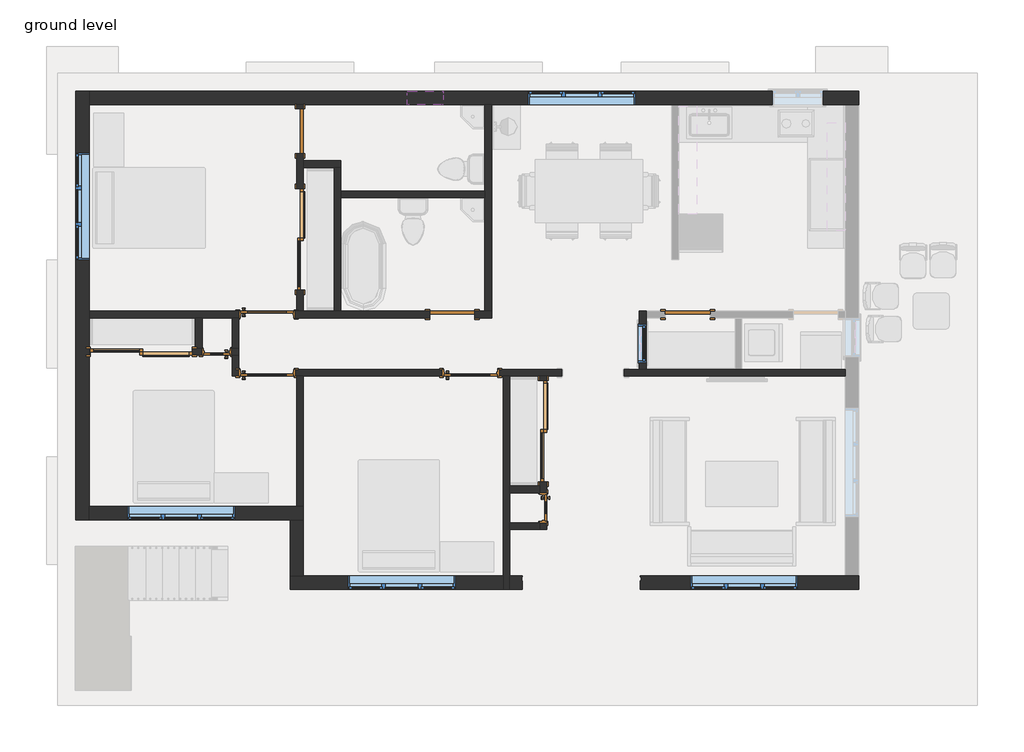
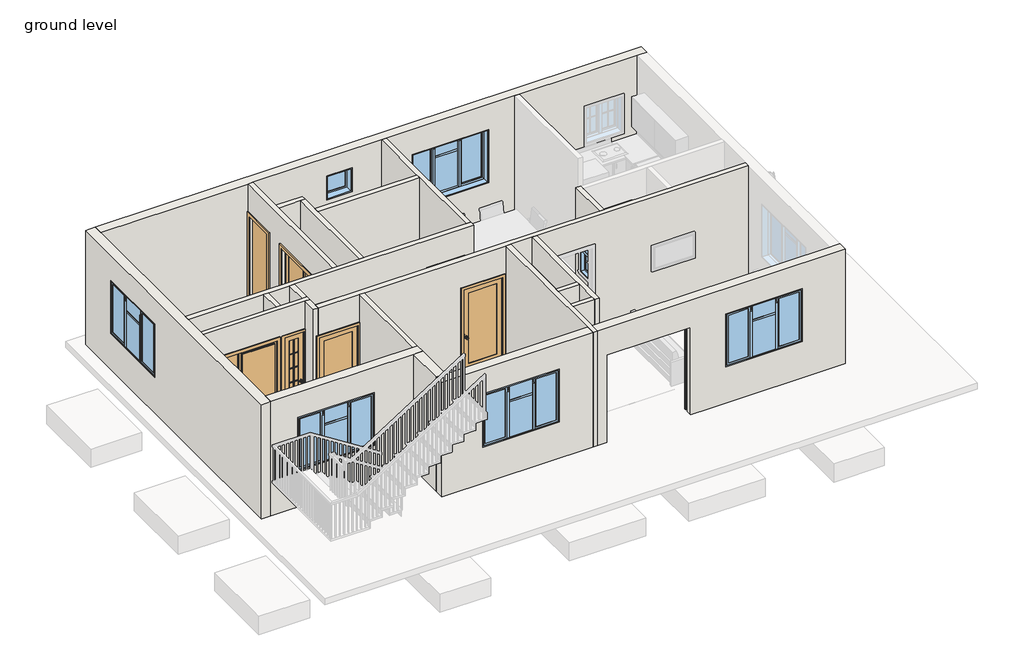
# One storey, part 1 of 4: 23 walls, 11 doors, 7 windows.
"""IFC4 building model written with IfcOpenShell, lengths in millimetres."""

from ifc_helpers import new_model, si_unit, frame, origin, place, context, project, spatial, polyline, outline, extrude, faceted_brep, transform, mapped, element, save
from components import door_505787c2, door_a3feeac7, door_3c6ab76a, door_ccf0cbd1, door_214872d5, door_78caadf7, window_80340324, window_7a1f68bc, window_d2058a86

model = new_model("IFC4")

# Units and contexts
model_context = context("Model", 3, world=origin())
ifc_project = project(units=[si_unit("LENGTHUNIT", "METRE", prefix="MILLI")], contexts=[model_context])

# Site, building, storey
site = spatial("IfcSite", under=ifc_project)
building = spatial("IfcBuilding", under=site)
storey = spatial("IfcBuildingStorey", under=building, Name="ground level", Elevation=609.6)

# Doors
placement = place(None, origin())
door_shape = door_505787c2(model_context)
element("IfcDoor", 1, ObjectType="Door-Double-Sliding : 68\" x 84\"", at=placement, inside=storey, context=model_context, shape_type="MappedRepresentation", body=[
    mapped(door_shape, transform((-1350.0263529, 910.5161978, 609.6), x_axis=(0.0, -1.0, 0.0), y_axis=(1.0, 0.0, 0.0), z_axis=(0.0, 0.0, 1.0))),
])
element("IfcDoor", 2, ObjectType="Door-Double-Sliding : 68\" x 84\"", at=placement, inside=storey, context=model_context, shape_type="MappedRepresentation", body=[
    mapped(door_shape, transform((-8046.1013529, 2383.7161978, 609.6), x_axis=(-1.0, 0.0, 0.0), y_axis=(0.0, -1.0, 0.0), z_axis=(0.0, 0.0, 1.0))),
])
element("IfcDoor", 3, ObjectType="Door-Double-Sliding : 68\" x 84\"", at=placement, inside=storey, context=model_context, shape_type="MappedRepresentation", body=[
    mapped(door_shape, transform((-5477.5263529, 4168.0661978, 609.6), x_axis=(0.0, -1.0, 0.0), y_axis=(1.0, 0.0, 0.0), z_axis=(0.0, 0.0, 1.0))),
])
door_2_shape = door_a3feeac7(model_context)
element("IfcDoor", 4, ObjectType="Door-Interior-Single-1_Panel-Wood : 36\" x 84\"", at=placement, inside=storey, context=model_context, shape_type="MappedRepresentation", body=[
    mapped(door_2_shape, transform((-5912.5013529, 1897.9411978, 609.6), x_axis=(1.0, 0.0, 0.0), y_axis=(0.0, 1.0, 0.0), z_axis=(0.0, 0.0, 1.0))),
])
element("IfcDoor", 5, ObjectType="Door-Interior-Single-1_Panel-Wood : 36\" x 84\"", at=placement, inside=storey, context=model_context, shape_type="MappedRepresentation", body=[
    mapped(door_2_shape, transform((-2454.9263529, 1897.9411978, 609.6), x_axis=(1.0, 0.0, 0.0), y_axis=(0.0, 1.0, 0.0), z_axis=(0.0, 0.0, 1.0))),
])
door_3_shape = door_3c6ab76a(model_context)
element("IfcDoor", 6, ObjectType="Door-Interior-Single-1_Panel-Wood : 36\" x 84\"", at=placement, inside=storey, context=model_context, shape_type="MappedRepresentation", body=[
    mapped(door_3_shape, transform((-5912.5013529, 2894.8911978, 609.6), x_axis=(1.0, 0.0, 0.0), y_axis=(0.0, 1.0, 0.0), z_axis=(0.0, 0.0, 1.0))),
])
door_4_shape = door_ccf0cbd1(model_context)
element("IfcDoor", 7, ObjectType="Door-Interior-Single-Full Glass-Wood : 18\" x 84\"", at=placement, inside=storey, context=model_context, shape_type="MappedRepresentation", body=[
    mapped(door_4_shape, transform((-1219.8513529, -391.2338022, 609.6), x_axis=(0.0, -1.0, 0.0), y_axis=(1.0, 0.0, 0.0), z_axis=(0.0, 0.0, 1.0))),
])
element("IfcDoor", 8, ObjectType="Door-Interior-Single-Full Glass-Wood : 18\" x 84\"", at=placement, inside=storey, context=model_context, shape_type="MappedRepresentation", body=[
    mapped(door_4_shape, transform((-6766.5763529, 2253.5411978, 609.6), x_axis=(-1.0, 0.0, 0.0), y_axis=(0.0, -1.0, 0.0), z_axis=(0.0, 0.0, 1.0))),
])
door_5_shape = door_214872d5(model_context)
element("IfcDoor", 9, ObjectType="Single-Flush : 30\" x 84\"", at=placement, inside=storey, context=model_context, shape_type="MappedRepresentation", body=[
    mapped(door_5_shape, transform((-2766.0763529, 2891.7161978, 609.6), x_axis=(1.0, 0.0, 0.0), y_axis=(0.0, 1.0, 0.0), z_axis=(0.0, 0.0, 1.0))),
])
element("IfcDoor", 10, ObjectType="Single-Flush : 30\" x 84\"", at=placement, inside=storey, context=model_context, shape_type="MappedRepresentation", body=[
    mapped(door_5_shape, transform((1228.0736471, 2891.7161978, 609.6), x_axis=(1.0, 0.0, 0.0), y_axis=(0.0, 1.0, 0.0), z_axis=(0.0, 0.0, 1.0))),
])
door_6_shape = door_78caadf7(model_context)
element("IfcDoor", 11, ObjectType="Single-Flush : 30\" x 84\"", at=placement, inside=storey, context=model_context, shape_type="MappedRepresentation", body=[
    mapped(door_6_shape, transform((-5350.5263529, 6006.3911978, 609.6), x_axis=(0.0, 1.0, 0.0), y_axis=(-1.0, 0.0, 0.0), z_axis=(0.0, 0.0, 1.0))),
])

# Walls
element("IfcWall", 12, ObjectType="Generic - 4.5\"", at=placement, inside=storey, context=model_context, shape_type="Brep", body=[
    faceted_brep([(-5407.6763529, 6454.0661978, 609.6), (-5407.6763529, 6387.3911978, 609.6), (-5407.6763529, 6387.3911978, 2743.2), (-5407.6763529, 5625.3911978, 2743.2), (-5407.6763529, 5625.3911978, 609.6), (-5407.6763529, 5031.6661978, 609.6), (-5407.6763529, 5031.6661978, 2743.2), (-5407.6763529, 3304.4661978, 2743.2), (-5407.6763529, 3304.4661978, 609.6), (-5407.6763529, 2948.8661978, 609.6), (-5407.6763529, 2948.8661978, 3505.2), (-5407.6763529, 6454.0661978, 3505.2), (-5293.3763529, 6387.3911978, 2743.2), (-5293.3763529, 6387.3911978, 609.6), (-5293.3763529, 6454.0661978, 609.6), (-5293.3763529, 6454.0661978, 3505.2), (-5293.3763529, 5501.5661978, 3505.2), (-5293.3763529, 5387.2661978, 3505.2), (-5293.3763529, 2948.8661978, 3505.2), (-5293.3763529, 2948.8661978, 609.6), (-5293.3763529, 3304.4661978, 609.6), (-5293.3763529, 3304.4661978, 2743.2), (-5293.3763529, 5031.6661978, 2743.2), (-5293.3763529, 5031.6661978, 609.6), (-5293.3763529, 5387.2661978, 609.6), (-5293.3763529, 5501.5661978, 609.6), (-5293.3763529, 5625.3911978, 609.6), (-5293.3763529, 5625.3911978, 2743.2)], [[[0, 1, 2, 3, 4, 5, 6, 7, 8, 9, 10, 11]], [[12, 13, 14, 15, 16, 17, 18, 19, 20, 21, 22, 23, 24, 25, 26, 27]], [[9, 8, 20, 19]], [[14, 13, 1, 0]], [[26, 25, 24, 23, 5, 4]], [[11, 10, 18, 17, 16, 15]], [[0, 11, 15, 14]], [[10, 9, 19, 18]], [[23, 22, 6, 5]], [[21, 20, 8, 7]], [[22, 21, 7, 6]], [[2, 1, 13, 12]], [[3, 2, 12, 27]], [[4, 3, 27, 26]]]),
])
element("IfcWall", 13, ObjectType="Generic - 4.5\"", at=placement, inside=storey, context=model_context, shape_type="Brep", body=[
    faceted_brep([(-2099.3263529, 2948.8661978, 609.6), (-2213.6263529, 2948.8661978, 609.6), (-2385.0763529, 2948.8661978, 609.6), (-2385.0763529, 2948.8661978, 2743.2), (-3147.0763529, 2948.8661978, 2743.2), (-3147.0763529, 2948.8661978, 609.6), (-4658.3763529, 2948.8661978, 609.6), (-4772.6763529, 2948.8661978, 609.6), (-5293.3763529, 2948.8661978, 609.6), (-5407.6763529, 2948.8661978, 609.6), (-5429.9013529, 2948.8661978, 609.6), (-5429.9013529, 2948.8661978, 2768.6), (-6395.1013529, 2948.8661978, 2768.6), (-6395.1013529, 2948.8661978, 609.6), (-8931.9263529, 2948.8661978, 609.6), (-8931.9263529, 2948.8661978, 3505.2), (-5407.6763529, 2948.8661978, 3505.2), (-5293.3763529, 2948.8661978, 3505.2), (-4772.6763529, 2948.8661978, 3505.2), (-4658.3763529, 2948.8661978, 3505.2), (-2213.6263529, 2948.8661978, 3505.2), (-2099.3263529, 2948.8661978, 3505.2), (-2385.0763529, 2834.5661978, 2743.2), (-2385.0763529, 2834.5661978, 609.6), (-2099.3263529, 2834.5661978, 609.6), (-2099.3263529, 2834.5661978, 3505.2), (-6391.9263529, 2834.5661978, 3505.2), (-6506.2263529, 2834.5661978, 3505.2), (-7014.2263529, 2834.5661978, 3505.2), (-7128.5263529, 2834.5661978, 3505.2), (-8931.9263529, 2834.5661978, 3505.2), (-8931.9263529, 2834.5661978, 609.6), (-7128.5263529, 2834.5661978, 609.6), (-7014.2263529, 2834.5661978, 609.6), (-6506.2263529, 2834.5661978, 609.6), (-6395.1013529, 2834.5661978, 609.6), (-6395.1013529, 2834.5661978, 2768.6), (-5429.9013529, 2834.5661978, 2768.6), (-5429.9013529, 2834.5661978, 609.6), (-3147.0763529, 2834.5661978, 609.6), (-3147.0763529, 2834.5661978, 2743.2)], [[[0, 1, 2, 3, 4, 5, 6, 7, 8, 9, 10, 11, 12, 13, 14, 15, 16, 17, 18, 19, 20, 21]], [[22, 23, 24, 25, 26, 27, 28, 29, 30, 31, 32, 33, 34, 35, 36, 37, 38, 39, 40]], [[31, 14, 13, 35, 34, 33, 32]], [[39, 38, 10, 9, 8, 7, 6, 5]], [[24, 23, 2, 1, 0]], [[21, 20, 19, 18, 17, 16, 15, 30, 29, 28, 27, 26, 25]], [[15, 14, 31, 30]], [[0, 21, 25, 24]], [[37, 11, 10, 38]], [[11, 37, 36, 12]], [[12, 36, 35, 13]], [[3, 2, 23, 22]], [[4, 3, 22, 40]], [[5, 4, 40, 39]]]),
])
element("IfcWall", 14, ObjectType="Generic - 4.5\"", at=placement, inside=storey, context=model_context, shape_type="Brep", body=[
    faceted_brep([(-8931.9263529, 2199.5661978, 609.6), (-8909.7013529, 2199.5661978, 609.6), (-8909.7013529, 2199.5661978, 2743.2), (-7182.5013529, 2199.5661978, 2743.2), (-7182.5013529, 2199.5661978, 609.6), (-7020.5763529, 2199.5661978, 609.6), (-7020.5763529, 2199.5661978, 2768.6), (-6512.5763529, 2199.5661978, 2768.6), (-6512.5763529, 2199.5661978, 609.6), (-6506.2263529, 2199.5661978, 609.6), (-6391.9263529, 2199.5661978, 609.6), (-6391.9263529, 2199.5661978, 3505.2), (-6506.2263529, 2199.5661978, 3505.2), (-8931.9263529, 2199.5661978, 3505.2), (-8909.7013529, 2313.8661978, 2743.2), (-8909.7013529, 2313.8661978, 609.6), (-8931.9263529, 2313.8661978, 609.6), (-8931.9263529, 2313.8661978, 3505.2), (-7128.5263529, 2313.8661978, 3505.2), (-7014.2263529, 2313.8661978, 3505.2), (-6506.2263529, 2313.8661978, 3505.2), (-6391.9263529, 2313.8661978, 3505.2), (-6391.9263529, 2313.8661978, 609.6), (-6506.2263529, 2313.8661978, 609.6), (-6512.5763529, 2313.8661978, 609.6), (-6512.5763529, 2313.8661978, 2768.6), (-7020.5763529, 2313.8661978, 2768.6), (-7020.5763529, 2313.8661978, 609.6), (-7128.5263529, 2313.8661978, 609.6), (-7182.5013529, 2313.8661978, 609.6), (-7182.5013529, 2313.8661978, 2743.2)], [[[0, 1, 2, 3, 4, 5, 6, 7, 8, 9, 10, 11, 12, 13]], [[14, 15, 16, 17, 18, 19, 20, 21, 22, 23, 24, 25, 26, 27, 28, 29, 30]], [[22, 10, 9, 8, 24, 23]], [[16, 15, 1, 0]], [[29, 28, 27, 5, 4]], [[13, 12, 11, 21, 20, 19, 18, 17]], [[0, 13, 17, 16]], [[11, 10, 22, 21]], [[26, 6, 5, 27]], [[6, 26, 25, 7]], [[7, 25, 24, 8]], [[4, 3, 30, 29]], [[2, 1, 15, 14]], [[3, 2, 14, 30]]]),
])
element("IfcWall", 15, ObjectType="Generic - 4.5\"", at=placement, inside=storey, context=model_context, shape_type="Brep", body=[
    faceted_brep([(-7014.2263529, 2313.8661978, 609.6), (-7014.2263529, 2834.5661978, 609.6), (-7014.2263529, 2834.5661978, 3505.2), (-7014.2263529, 2313.8661978, 3505.2), (-7128.5263529, 2313.8661978, 609.6), (-7128.5263529, 2313.8661978, 3505.2), (-7128.5263529, 2834.5661978, 3505.2), (-7128.5263529, 2834.5661978, 609.6), (-7020.5763529, 2313.8661978, 609.6)], [[[0, 1, 2, 3]], [[4, 5, 6, 7]], [[1, 0, 8, 4, 7]], [[3, 2, 6, 5]], [[0, 3, 5, 4, 8]], [[2, 1, 7, 6]]]),
])
element("IfcWall", 16, ObjectType="Generic - 4.5\"", at=placement, inside=storey, context=model_context, shape_type="Brep", body=[
    faceted_brep([(-6391.9263529, 2313.8661978, 609.6), (-6391.9263529, 2834.5661978, 609.6), (-6391.9263529, 2834.5661978, 3505.2), (-6391.9263529, 2313.8661978, 3505.2), (-6506.2263529, 2313.8661978, 609.6), (-6506.2263529, 2313.8661978, 3505.2), (-6506.2263529, 2834.5661978, 3505.2), (-6506.2263529, 2834.5661978, 609.6), (-6395.1013529, 2834.5661978, 609.6)], [[[0, 1, 2, 3]], [[4, 5, 6, 7]], [[1, 0, 4, 7, 8]], [[3, 2, 6, 5]], [[0, 3, 5, 4]], [[2, 1, 8, 7, 6]]]),
])
element("IfcWall", 17, ObjectType="Generic - 4.5\"", at=placement, inside=storey, context=model_context, shape_type="SweptSolid", body=[
    extrude(outline(polyline([(-5293.3763529, 1843.9661978), (-5293.3763529, -365.8338022), (-5407.6763529, -365.8338022), (-5407.6763529, 1843.9661978), (-5293.3763529, 1843.9661978)])), frame((0.0, 0.0, 609.6), z_axis=(0.0, 0.0, 1.0), x_axis=(1.0, 0.0, 0.0)), (0.0, 0.0, 1.0), 2895.6),
])
element("IfcWall", 18, ObjectType="Generic - 4.5\"", at=placement, inside=storey, context=model_context, shape_type="Brep", body=[
    faceted_brep([(-6506.2263529, 2199.5661978, 609.6), (-6506.2263529, 1843.9661978, 609.6), (-6506.2263529, 1843.9661978, 3505.2), (-6506.2263529, 2199.5661978, 3505.2), (-6391.9263529, 2199.5661978, 3505.2), (-6391.9263529, 1958.2661978, 3505.2), (-6391.9263529, 1843.9661978, 3505.2), (-6391.9263529, 1843.9661978, 2768.6), (-6391.9263529, 1958.2661978, 2768.6), (-6391.9263529, 1958.2661978, 609.6), (-6391.9263529, 2199.5661978, 609.6), (-6395.1013529, 1958.2661978, 609.6), (-6395.1013529, 1843.9661978, 609.6), (-6395.1013529, 1843.9661978, 2768.6), (-6395.1013529, 1958.2661978, 2768.6)], [[[0, 1, 2, 3]], [[4, 5, 6, 7, 8, 9, 10]], [[1, 0, 10, 9, 11, 12]], [[3, 2, 6, 5, 4]], [[0, 3, 4, 10]], [[2, 1, 12, 13, 7, 6]], [[14, 11, 9, 8]], [[13, 14, 8, 7]], [[11, 14, 13, 12]]]),
])
element("IfcWall", 19, ObjectType="Generic - 4.5\"", at=placement, inside=storey, context=model_context, shape_type="Brep", body=[
    faceted_brep([(-1972.3263529, 1843.9661978, 609.6), (-1902.4763529, 1843.9661978, 609.6), (-1788.1763529, 1843.9661978, 609.6), (-1280.1763529, 1843.9661978, 609.6), (-1165.8763529, 1843.9661978, 609.6), (-911.8763529, 1843.9661978, 609.6), (-911.8763529, 1843.9661978, 2743.2), (154.9236471, 1843.9661978, 2743.2), (154.9236471, 1843.9661978, 609.6), (3901.4236471, 1843.9661978, 609.6), (3901.4236471, 1843.9661978, 3505.2), (-1165.8763529, 1843.9661978, 3505.2), (-1280.1763529, 1843.9661978, 3505.2), (-1788.1763529, 1843.9661978, 3505.2), (-1902.4763529, 1843.9661978, 3505.2), (-5293.3763529, 1843.9661978, 3505.2), (-5407.6763529, 1843.9661978, 3505.2), (-6391.9263529, 1843.9661978, 3505.2), (-6391.9263529, 1843.9661978, 2768.6), (-5429.9013529, 1843.9661978, 2768.6), (-5429.9013529, 1843.9661978, 609.6), (-5407.6763529, 1843.9661978, 609.6), (-5293.3763529, 1843.9661978, 609.6), (-2937.5263529, 1843.9661978, 609.6), (-2937.5263529, 1843.9661978, 2768.6), (-1972.3263529, 1843.9661978, 2768.6), (-911.8763529, 1958.2661978, 2743.2), (-911.8763529, 1958.2661978, 609.6), (-1972.3263529, 1958.2661978, 609.6), (-1972.3263529, 1958.2661978, 2768.6), (-2937.5263529, 1958.2661978, 2768.6), (-2937.5263529, 1958.2661978, 609.6), (-5429.9013529, 1958.2661978, 609.6), (-5429.9013529, 1958.2661978, 2768.6), (-6391.9263529, 1958.2661978, 2768.6), (-6391.9263529, 1958.2661978, 3505.2), (408.9236471, 1958.2661978, 3505.2), (523.2236471, 1958.2661978, 3505.2), (2034.5236471, 1958.2661978, 3505.2), (2148.8236471, 1958.2661978, 3505.2), (3901.4236471, 1958.2661978, 3505.2), (3901.4236471, 1958.2661978, 609.6), (2148.8236471, 1958.2661978, 609.6), (2034.5236471, 1958.2661978, 609.6), (523.2236471, 1958.2661978, 609.6), (408.9236471, 1958.2661978, 609.6), (154.9236471, 1958.2661978, 609.6), (154.9236471, 1958.2661978, 2743.2)], [[[0, 1, 2, 3, 4, 5, 6, 7, 8, 9, 10, 11, 12, 13, 14, 15, 16, 17, 18, 19, 20, 21, 22, 23, 24, 25]], [[26, 27, 28, 29, 30, 31, 32, 33, 34, 35, 36, 37, 38, 39, 40, 41, 42, 43, 44, 45, 46, 47]], [[20, 32, 31, 23, 22, 21]], [[28, 27, 5, 4, 3, 2, 1, 0]], [[46, 45, 44, 43, 42, 41, 9, 8]], [[17, 16, 15, 14, 13, 12, 11, 10, 40, 39, 38, 37, 36, 35]], [[17, 35, 34, 18]], [[10, 9, 41, 40]], [[19, 18, 34, 33]], [[25, 29, 28, 0]], [[29, 25, 24, 30]], [[30, 24, 23, 31]], [[19, 33, 32, 20]], [[8, 7, 47, 46]], [[6, 5, 27, 26]], [[7, 6, 26, 47]]]),
])
element("IfcWall", 20, ObjectType="Generic - 4.5\"", at=placement, inside=storey, context=model_context, shape_type="Brep", body=[
    faceted_brep([(-1902.4763529, 1843.9661978, 609.6), (-1902.4763529, -1546.9338022, 609.6), (-1902.4763529, -1775.5338022, 609.6), (-1902.4763529, -1775.5338022, 3505.2), (-1902.4763529, -1546.9338022, 3505.2), (-1902.4763529, 1843.9661978, 3505.2), (-1788.1763529, 1843.9661978, 609.6), (-1788.1763529, 1843.9661978, 3505.2), (-1788.1763529, -22.9338022, 3505.2), (-1788.1763529, -137.2338022, 3505.2), (-1788.1763529, -645.2338022, 3505.2), (-1788.1763529, -759.5338022, 3505.2), (-1788.1763529, -1546.9338022, 3505.2), (-1788.1763529, -1775.5338022, 3505.2), (-1788.1763529, -1775.5338022, 609.6), (-1788.1763529, -1546.9338022, 609.6), (-1788.1763529, -759.5338022, 609.6), (-1788.1763529, -645.2338022, 609.6), (-1788.1763529, -137.2338022, 609.6), (-1788.1763529, -22.9338022, 609.6)], [[[0, 1, 2, 3, 4, 5]], [[6, 7, 8, 9, 10, 11, 12, 13, 14, 15, 16, 17, 18, 19]], [[2, 1, 0, 6, 19, 18, 17, 16, 15, 14]], [[5, 4, 3, 13, 12, 11, 10, 9, 8, 7]], [[0, 5, 7, 6]], [[3, 2, 14, 13]]]),
])
element("IfcWall", 21, ObjectType="Generic - 4.5\"", at=placement, inside=storey, context=model_context, shape_type="Brep", body=[
    faceted_brep([(-1280.1763529, 46.9161978, 2743.2), (-1280.1763529, 46.9161978, 609.6), (-1280.1763529, -22.9338022, 609.6), (-1280.1763529, -137.2338022, 609.6), (-1280.1763529, -137.2338022, 2768.6), (-1280.1763529, -645.2338022, 2768.6), (-1280.1763529, -645.2338022, 609.6), (-1280.1763529, -759.5338022, 609.6), (-1280.1763529, -759.5338022, 3505.2), (-1280.1763529, -645.2338022, 3505.2), (-1280.1763529, -137.2338022, 3505.2), (-1280.1763529, -22.9338022, 3505.2), (-1280.1763529, 1843.9661978, 3505.2), (-1280.1763529, 1843.9661978, 609.6), (-1280.1763529, 1774.1161978, 609.6), (-1280.1763529, 1774.1161978, 2743.2), (-1165.8763529, -137.2338022, 609.6), (-1165.8763529, 46.9161978, 609.6), (-1165.8763529, 46.9161978, 2743.2), (-1165.8763529, 1774.1161978, 2743.2), (-1165.8763529, 1774.1161978, 609.6), (-1165.8763529, 1843.9661978, 609.6), (-1165.8763529, 1843.9661978, 3505.2), (-1165.8763529, -759.5338022, 3505.2), (-1165.8763529, -759.5338022, 609.6), (-1165.8763529, -645.2338022, 609.6), (-1165.8763529, -645.2338022, 2768.6), (-1165.8763529, -137.2338022, 2768.6)], [[[0, 1, 2, 3, 4, 5, 6, 7, 8, 9, 10, 11, 12, 13, 14, 15]], [[16, 17, 18, 19, 20, 21, 22, 23, 24, 25, 26, 27]], [[24, 7, 6, 25]], [[14, 13, 21, 20]], [[3, 2, 1, 17, 16]], [[12, 11, 10, 9, 8, 23, 22]], [[13, 12, 22, 21]], [[8, 7, 24, 23]], [[5, 26, 25, 6]], [[26, 5, 4, 27]], [[27, 4, 3, 16]], [[20, 19, 15, 14]], [[18, 17, 1, 0]], [[19, 18, 0, 15]]]),
])
element("IfcWall", 22, ObjectType="Generic - 4.5\"", at=placement, inside=storey, context=model_context, shape_type="Brep", body=[
    faceted_brep([(-1280.1763529, -22.9338022, 609.6), (-1788.1763529, -22.9338022, 609.6), (-1788.1763529, -22.9338022, 3505.2), (-1280.1763529, -22.9338022, 3505.2), (-1280.1763529, -137.2338022, 609.6), (-1280.1763529, -137.2338022, 2768.6), (-1280.1763529, -137.2338022, 3505.2), (-1788.1763529, -137.2338022, 3505.2), (-1788.1763529, -137.2338022, 609.6)], [[[0, 1, 2, 3]], [[4, 5, 6, 7, 8]], [[1, 0, 4, 8]], [[3, 2, 7, 6]], [[0, 3, 6, 5, 4]], [[2, 1, 8, 7]]]),
])
element("IfcWall", 23, ObjectType="Generic - 4.5\"", at=placement, inside=storey, context=model_context, shape_type="SweptSolid", body=[
    extrude(outline(polyline([(-1788.1763529, -645.2338022), (-1280.1763529, -645.2338022), (-1280.1763529, -759.5338022), (-1788.1763529, -759.5338022), (-1788.1763529, -645.2338022)])), frame((0.0, 0.0, 609.6), z_axis=(0.0, 0.0, 1.0), x_axis=(1.0, 0.0, 0.0)), (0.0, 0.0, 1.0), 2895.6),
])
element("IfcWall", 24, ObjectType="Generic - 4.5\"", at=placement, inside=storey, context=model_context, shape_type="Brep", body=[
    faceted_brep([(-2099.3263529, 2948.8661978, 609.6), (-2099.3263529, 6454.0661978, 609.6), (-2099.3263529, 6454.0661978, 3505.2), (-2099.3263529, 2948.8661978, 3505.2), (-2213.6263529, 2948.8661978, 609.6), (-2213.6263529, 2948.8661978, 3505.2), (-2213.6263529, 4872.9161978, 3505.2), (-2213.6263529, 4987.2161978, 3505.2), (-2213.6263529, 6454.0661978, 3505.2), (-2213.6263529, 6454.0661978, 609.6), (-2213.6263529, 4987.2161978, 609.6), (-2213.6263529, 4872.9161978, 609.6)], [[[0, 1, 2, 3]], [[4, 5, 6, 7, 8, 9, 10, 11]], [[1, 0, 4, 11, 10, 9]], [[3, 2, 8, 7, 6, 5]], [[2, 1, 9, 8]], [[0, 3, 5, 4]]]),
])
element("IfcWall", 25, ObjectType="Generic - 4.5\"", at=placement, inside=storey, context=model_context, shape_type="Brep", body=[
    faceted_brep([(-5293.3763529, 5387.2661978, 609.6), (-4772.6763529, 5387.2661978, 609.6), (-4658.3763529, 5387.2661978, 609.6), (-4658.3763529, 5387.2661978, 3505.2), (-4772.6763529, 5387.2661978, 3505.2), (-5293.3763529, 5387.2661978, 3505.2), (-5293.3763529, 5501.5661978, 609.6), (-5293.3763529, 5501.5661978, 3505.2), (-4658.3763529, 5501.5661978, 3505.2), (-4658.3763529, 5501.5661978, 609.6)], [[[0, 1, 2, 3, 4, 5]], [[6, 7, 8, 9]], [[2, 1, 0, 6, 9]], [[5, 4, 3, 8, 7]], [[0, 5, 7, 6]], [[3, 2, 9, 8]]]),
])
element("IfcWall", 26, ObjectType="Generic - 4.5\"", at=placement, inside=storey, context=model_context, shape_type="Brep", body=[
    faceted_brep([(-4772.6763529, 5387.2661978, 609.6), (-4772.6763529, 2948.8661978, 609.6), (-4772.6763529, 2948.8661978, 3505.2), (-4772.6763529, 5387.2661978, 3505.2), (-4658.3763529, 5387.2661978, 609.6), (-4658.3763529, 5387.2661978, 3505.2), (-4658.3763529, 4987.2161978, 3505.2), (-4658.3763529, 4872.9161978, 3505.2), (-4658.3763529, 2948.8661978, 3505.2), (-4658.3763529, 2948.8661978, 609.6), (-4658.3763529, 4872.9161978, 609.6), (-4658.3763529, 4987.2161978, 609.6)], [[[0, 1, 2, 3]], [[4, 5, 6, 7, 8, 9, 10, 11]], [[1, 0, 4, 11, 10, 9]], [[3, 2, 8, 7, 6, 5]], [[0, 3, 5, 4]], [[2, 1, 9, 8]]]),
])
element("IfcWall", 27, ObjectType="Generic - 4.5\"", at=placement, inside=storey, context=model_context, shape_type="SweptSolid", body=[
    extrude(outline(polyline([(-4658.3763529, 4987.2161978), (-2213.6263529, 4987.2161978), (-2213.6263529, 4872.9161978), (-4658.3763529, 4872.9161978), (-4658.3763529, 4987.2161978)])), frame((0.0, 0.0, 609.6), z_axis=(0.0, 0.0, 1.0), x_axis=(1.0, 0.0, 0.0)), (0.0, 0.0, 1.0), 2895.6),
])
element("IfcWall", 28, ObjectType="Generic - 4.5\"", at=placement, inside=storey, context=model_context, shape_type="Brep", body=[
    faceted_brep([(523.2236471, 1958.2661978, 609.6), (523.2236471, 2834.5661978, 609.6), (523.2236471, 2948.8661978, 609.6), (523.2236471, 2948.8661978, 3505.2), (523.2236471, 2834.5661978, 3505.2), (523.2236471, 1958.2661978, 3505.2), (523.2236471, 2726.6161978, 2590.8), (523.2236471, 2726.6161978, 1524.0), (523.2236471, 2066.2161978, 1524.0), (523.2236471, 2066.2161978, 2590.8), (408.9236471, 1958.2661978, 609.6), (408.9236471, 1958.2661978, 3505.2), (408.9236471, 2948.8661978, 3505.2), (408.9236471, 2948.8661978, 609.6), (408.9236471, 2726.6161978, 2590.8), (408.9236471, 2066.2161978, 2590.8), (408.9236471, 2066.2161978, 1524.0), (408.9236471, 2726.6161978, 1524.0)], [[[0, 1, 2, 3, 4, 5], [6, 7, 8, 9]], [[10, 11, 12, 13], [14, 15, 16, 17]], [[2, 1, 0, 10, 13]], [[5, 4, 3, 12, 11]], [[0, 5, 11, 10]], [[3, 2, 13, 12]], [[7, 6, 14, 17]], [[8, 7, 17, 16]], [[9, 8, 16, 15]], [[6, 9, 15, 14]]]),
])
element("IfcWall", 29, ObjectType="Generic - 9\"", at=placement, inside=storey, context=model_context, shape_type="Brep", body=[
    faceted_brep([(-9160.5263529, 6682.6661978, 609.6), (-9160.5263529, -594.4338022, 609.6), (-9160.5263529, -594.4338022, 3505.2), (-9160.5263529, 6682.6661978, 3505.2), (-9160.5263529, 5644.4411978, 2870.2), (-9160.5263529, 3815.6411978, 2870.2), (-9160.5263529, 3815.6411978, 1524.0), (-9160.5263529, 5644.4411978, 1524.0), (-8931.9263529, 6682.6661978, 609.6), (-8931.9263529, 6682.6661978, 3505.2), (-8931.9263529, 6454.0661978, 3505.2), (-8931.9263529, 2948.8661978, 3505.2), (-8931.9263529, 2834.5661978, 3505.2), (-8931.9263529, 2313.8661978, 3505.2), (-8931.9263529, 2199.5661978, 3505.2), (-8931.9263529, -365.8338022, 3505.2), (-8931.9263529, -594.4338022, 3505.2), (-8931.9263529, -594.4338022, 609.6), (-8931.9263529, -365.8338022, 609.6), (-8931.9263529, 2199.5661978, 609.6), (-8931.9263529, 2313.8661978, 609.6), (-8931.9263529, 2834.5661978, 609.6), (-8931.9263529, 2948.8661978, 609.6), (-8931.9263529, 6454.0661978, 609.6), (-8931.9263529, 5644.4411978, 2870.2), (-8931.9263529, 5644.4411978, 1524.0), (-8931.9263529, 3815.6411978, 1524.0), (-8931.9263529, 3815.6411978, 2870.2)], [[[0, 1, 2, 3], [4, 5, 6, 7]], [[8, 9, 10, 11, 12, 13, 14, 15, 16, 17, 18, 19, 20, 21, 22, 23], [24, 25, 26, 27]], [[1, 0, 8, 23, 22, 21, 20, 19, 18, 17]], [[3, 2, 16, 15, 14, 13, 12, 11, 10, 9]], [[0, 3, 9, 8]], [[2, 1, 17, 16]], [[25, 24, 4, 7]], [[26, 25, 7, 6]], [[27, 26, 6, 5]], [[24, 27, 5, 4]]]),
])
element("IfcWall", 30, ObjectType="Generic - 9\"", at=placement, inside=storey, context=model_context, shape_type="Brep", body=[
    faceted_brep([(-8931.9263529, 6454.0661978, 609.6), (-5407.6763529, 6454.0661978, 609.6), (-5293.3763529, 6454.0661978, 609.6), (-2213.6263529, 6454.0661978, 609.6), (-2099.3263529, 6454.0661978, 609.6), (961.3736471, 6454.0661978, 609.6), (1075.6736471, 6454.0661978, 609.6), (3901.4236471, 6454.0661978, 609.6), (4130.0236471, 6454.0661978, 609.6), (4130.0236471, 6454.0661978, 3505.2), (3901.4236471, 6454.0661978, 3505.2), (1075.6736471, 6454.0661978, 3505.2), (961.3736471, 6454.0661978, 3505.2), (-2099.3263529, 6454.0661978, 3505.2), (-2213.6263529, 6454.0661978, 3505.2), (-5293.3763529, 6454.0661978, 3505.2), (-5407.6763529, 6454.0661978, 3505.2), (-8931.9263529, 6454.0661978, 3505.2), (3533.1236471, 6454.0661978, 2616.2), (3533.1236471, 6454.0661978, 1701.8), (2669.5236471, 6454.0661978, 1701.8), (2669.5236471, 6454.0661978, 2616.2), (345.4236471, 6454.0661978, 2870.2), (345.4236471, 6454.0661978, 1524.0), (-1483.3763529, 6454.0661978, 1524.0), (-1483.3763529, 6454.0661978, 2870.2), (-2918.4763529, 6454.0661978, 3048.0), (-2918.4763529, 6454.0661978, 2438.4), (-3528.0763529, 6454.0661978, 2438.4), (-3528.0763529, 6454.0661978, 3048.0), (-8931.9263529, 6682.6661978, 609.6), (-8931.9263529, 6682.6661978, 3505.2), (4130.0236471, 6682.6661978, 3505.2), (4130.0236471, 6682.6661978, 609.6), (3533.1236471, 6682.6661978, 2616.2), (2669.5236471, 6682.6661978, 2616.2), (2669.5236471, 6682.6661978, 1701.8), (3533.1236471, 6682.6661978, 1701.8), (345.4236471, 6682.6661978, 2870.2), (-1483.3763529, 6682.6661978, 2870.2), (-1483.3763529, 6682.6661978, 1524.0), (345.4236471, 6682.6661978, 1524.0), (-2918.4763529, 6682.6661978, 3048.0), (-3528.0763529, 6682.6661978, 3048.0), (-3528.0763529, 6682.6661978, 2438.4), (-2918.4763529, 6682.6661978, 2438.4)], [[[0, 1, 2, 3, 4, 5, 6, 7, 8, 9, 10, 11, 12, 13, 14, 15, 16, 17], [18, 19, 20, 21], [22, 23, 24, 25], [26, 27, 28, 29]], [[30, 31, 32, 33], [34, 35, 36, 37], [38, 39, 40, 41], [42, 43, 44, 45]], [[8, 7, 6, 5, 4, 3, 2, 1, 0, 30, 33]], [[17, 16, 15, 14, 13, 12, 11, 10, 9, 32, 31]], [[0, 17, 31, 30]], [[9, 8, 33, 32]], [[19, 18, 34, 37]], [[20, 19, 37, 36]], [[21, 20, 36, 35]], [[18, 21, 35, 34]], [[23, 22, 38, 41]], [[24, 23, 41, 40]], [[25, 24, 40, 39]], [[22, 25, 39, 38]], [[27, 26, 42, 45]], [[28, 27, 45, 44]], [[29, 28, 44, 43]], [[26, 29, 43, 42]]]),
])
element("IfcWall", 31, ObjectType="Generic - 9\"", at=placement, inside=storey, context=model_context, shape_type="Brep", body=[
    faceted_brep([(-8931.9263529, -594.4338022, 609.6), (-5521.9763529, -594.4338022, 609.6), (-5293.3763529, -594.4338022, 609.6), (-5293.3763529, -594.4338022, 3505.2), (-5521.9763529, -594.4338022, 3505.2), (-8931.9263529, -594.4338022, 3505.2), (-8284.2263529, -594.4338022, 2870.2), (-6455.4263529, -594.4338022, 2870.2), (-6455.4263529, -594.4338022, 1524.0), (-8284.2263529, -594.4338022, 1524.0), (-8931.9263529, -365.8338022, 609.6), (-8931.9263529, -365.8338022, 3505.2), (-5407.6763529, -365.8338022, 3505.2), (-5293.3763529, -365.8338022, 3505.2), (-5293.3763529, -365.8338022, 609.6), (-5407.6763529, -365.8338022, 609.6), (-8284.2263529, -365.8338022, 2870.2), (-8284.2263529, -365.8338022, 1524.0), (-6455.4263529, -365.8338022, 1524.0), (-6455.4263529, -365.8338022, 2870.2)], [[[0, 1, 2, 3, 4, 5], [6, 7, 8, 9]], [[10, 11, 12, 13, 14, 15], [16, 17, 18, 19]], [[2, 1, 0, 10, 15, 14]], [[5, 4, 3, 13, 12, 11]], [[3, 2, 14, 13]], [[0, 5, 11, 10]], [[17, 16, 6, 9]], [[18, 17, 9, 8]], [[19, 18, 8, 7]], [[16, 19, 7, 6]]]),
])
element("IfcWall", 32, ObjectType="Generic - 9\"", at=placement, inside=storey, context=model_context, shape_type="Brep", body=[
    faceted_brep([(-1902.4763529, -1546.9338022, 609.6), (-5293.3763529, -1546.9338022, 609.6), (-5521.9763529, -1546.9338022, 609.6), (-5521.9763529, -1546.9338022, 3505.2), (-5293.3763529, -1546.9338022, 3505.2), (-1902.4763529, -1546.9338022, 3505.2), (-4540.9013529, -1546.9338022, 2870.2), (-4540.9013529, -1546.9338022, 1524.0), (-2712.1013529, -1546.9338022, 1524.0), (-2712.1013529, -1546.9338022, 2870.2), (-1902.4763529, -1775.5338022, 609.6), (-1902.4763529, -1775.5338022, 3505.2), (-5521.9763529, -1775.5338022, 3505.2), (-5521.9763529, -1775.5338022, 609.6), (-4540.9013529, -1775.5338022, 2870.2), (-2712.1013529, -1775.5338022, 2870.2), (-2712.1013529, -1775.5338022, 1524.0), (-4540.9013529, -1775.5338022, 1524.0)], [[[0, 1, 2, 3, 4, 5], [6, 7, 8, 9]], [[10, 11, 12, 13], [14, 15, 16, 17]], [[2, 1, 0, 10, 13]], [[5, 4, 3, 12, 11]], [[0, 5, 11, 10]], [[3, 2, 13, 12]], [[7, 6, 14, 17]], [[8, 7, 17, 16]], [[9, 8, 16, 15]], [[6, 9, 15, 14]]]),
])
element("IfcWall", 33, ObjectType="Generic - 9\"", at=placement, inside=storey, context=model_context, shape_type="SweptSolid", body=[
    extrude(outline(polyline([(-5521.9763529, -1546.9338022), (-5521.9763529, -594.4338022), (-5293.3763529, -594.4338022), (-5293.3763529, -1546.9338022), (-5521.9763529, -1546.9338022)])), frame((0.0, 0.0, 609.6), z_axis=(0.0, 0.0, 1.0), x_axis=(1.0, 0.0, 0.0)), (0.0, 0.0, 1.0), 2895.6),
])
element("IfcWall", 34, ObjectType="Generic - 9\"", at=placement, inside=storey, context=model_context, shape_type="Brep", body=[
    faceted_brep([(4130.0236471, -1775.5338022, 3505.2), (-1788.1763529, -1775.5338022, 3505.2), (-1788.1763529, -1775.5338022, 609.6), (-1575.3263529, -1775.5338022, 609.6), (-1575.3263529, -1775.5338022, 2818.6), (424.6736471, -1775.5338022, 2818.6), (424.6736471, -1775.5338022, 609.6), (4130.0236471, -1775.5338022, 609.6), (1272.5236471, -1775.5338022, 2870.2), (3101.3236471, -1775.5338022, 2870.2), (3101.3236471, -1775.5338022, 1524.0), (1272.5236471, -1775.5338022, 1524.0), (-1788.1763529, -1546.9338022, 3505.2), (3901.4236471, -1546.9338022, 3505.2), (4130.0236471, -1546.9338022, 3505.2), (4130.0236471, -1546.9338022, 609.6), (3901.4236471, -1546.9338022, 609.6), (424.6736471, -1546.9338022, 609.6), (424.6736471, -1546.9338022, 2818.6), (-1575.3263529, -1546.9338022, 2818.6), (-1575.3263529, -1546.9338022, 609.6), (-1788.1763529, -1546.9338022, 609.6), (1272.5236471, -1546.9338022, 2870.2), (1272.5236471, -1546.9338022, 1524.0), (3101.3236471, -1546.9338022, 1524.0), (3101.3236471, -1546.9338022, 2870.2), (-1575.3263529, -1566.9338022, 609.6), (-1590.3263529, -1566.9338022, 609.6), (-1590.3263529, -1636.9338022, 609.6), (-1575.3263529, -1636.9338022, 609.6), (424.6736471, -1636.9338022, 609.6), (439.6736471, -1636.9338022, 609.6), (439.6736471, -1566.9338022, 609.6), (424.6736471, -1566.9338022, 609.6), (424.6736471, -1566.9338022, 2818.6), (-1575.3263529, -1566.9338022, 2818.6), (-1575.3263529, -1636.9338022, 2818.6), (424.6736471, -1636.9338022, 2818.6), (-1590.3263529, -1636.9338022, 2833.6), (439.6736471, -1636.9338022, 2833.6), (439.6736471, -1566.9338022, 2833.6), (-1590.3263529, -1566.9338022, 2833.6)], [[[0, 1, 2, 3, 4, 5, 6, 7], [8, 9, 10, 11]], [[12, 13, 14, 15, 16, 17, 18, 19, 20, 21], [22, 23, 24, 25]], [[2, 21, 20, 26, 27, 28, 29, 3]], [[15, 7, 6, 30, 31, 32, 33, 17, 16]], [[1, 0, 14, 13, 12]], [[2, 1, 12, 21]], [[0, 7, 15, 14]], [[34, 35, 19, 18]], [[36, 37, 5, 4]], [[29, 36, 4, 3]], [[37, 30, 6, 5]], [[37, 36, 29, 28, 38, 39, 31, 30]], [[31, 39, 40, 32]], [[35, 34, 33, 32, 40, 41, 27, 26]], [[33, 34, 18, 17]], [[35, 26, 20, 19]], [[38, 28, 27, 41]], [[39, 38, 41, 40]], [[23, 22, 8, 11]], [[24, 23, 11, 10]], [[25, 24, 10, 9]], [[22, 25, 9, 8]]]),
])

# Windows
window_shape = window_80340324(model_context)
element("IfcWindow", 35, ObjectType="Fixed : 24\" x 24\"", at=placement, inside=storey, context=model_context, shape_type="MappedRepresentation", body=[
    mapped(window_shape, transform((-3185.1763529, 6568.3661978, 1524.0), x_axis=(1.0, 0.0, 0.0), y_axis=(0.0, 1.0, 0.0), z_axis=(0.0, 0.0, 1.0))),
])
window_2_shape = window_7a1f68bc(model_context)
element("IfcWindow", 36, ObjectType="Window-Casement-Triple-Middle-Transom : 72\" x 53\"", at=placement, inside=storey, context=model_context, shape_type="MappedRepresentation", body=[
    mapped(window_2_shape, transform((-3626.5013529, -1661.2338022, 609.6), x_axis=(-1.0, 0.0, 0.0), y_axis=(0.0, -1.0, 0.0), z_axis=(0.0, 0.0, 1.0))),
])
element("IfcWindow", 37, ObjectType="Window-Casement-Triple-Middle-Transom : 72\" x 53\"", at=placement, inside=storey, context=model_context, shape_type="MappedRepresentation", body=[
    mapped(window_2_shape, transform((-7369.8263529, -480.1338022, 609.6), x_axis=(-1.0, 0.0, 0.0), y_axis=(0.0, -1.0, 0.0), z_axis=(0.0, 0.0, 1.0))),
])
element("IfcWindow", 38, ObjectType="Window-Casement-Triple-Middle-Transom : 72\" x 53\"", at=placement, inside=storey, context=model_context, shape_type="MappedRepresentation", body=[
    mapped(window_2_shape, transform((-9046.2263529, 4730.0411978, 609.6), x_axis=(0.0, 1.0, 0.0), y_axis=(-1.0, 0.0, 0.0), z_axis=(0.0, 0.0, 1.0))),
])
element("IfcWindow", 39, ObjectType="Window-Casement-Triple-Middle-Transom : 72\" x 53\"", at=placement, inside=storey, context=model_context, shape_type="MappedRepresentation", body=[
    mapped(window_2_shape, transform((-568.9763529, 6568.3661978, 609.6), x_axis=(1.0, 0.0, 0.0), y_axis=(0.0, 1.0, 0.0), z_axis=(0.0, 0.0, 1.0))),
])
element("IfcWindow", 40, ObjectType="Window-Casement-Triple-Middle-Transom : 72\" x 53\"", at=placement, inside=storey, context=model_context, shape_type="MappedRepresentation", body=[
    mapped(window_2_shape, transform((2186.9236471, -1661.2338022, 609.6), x_axis=(-1.0, 0.0, 0.0), y_axis=(0.0, -1.0, 0.0), z_axis=(0.0, 0.0, 1.0))),
])
window_3_shape = window_d2058a86(model_context)
element("IfcWindow", 41, ObjectType="Window-Double-Hung : 26\" x 42\"", at=placement, inside=storey, context=model_context, shape_type="MappedRepresentation", body=[
    mapped(window_3_shape, transform((466.0736471, 2396.4161978, 609.6), x_axis=(0.0, -1.0, 0.0), y_axis=(1.0, 0.0, 0.0), z_axis=(0.0, 0.0, 1.0))),
])

save(model, "model.ifc")

# Revit data of these elements
# Type "Door-Double-Sliding : 68\" x 84\""
#   Type Mark = "14"
#   Construction Type Id = "opn-d45"
#   Assembly Code = "C1020"
#   Analytic Construction = "Wood frame, double glass door "
#   Thickness = 0' - 2"
#   Thermal Resistance (R) = 1.8150 (h·ft²·°F)/BTU
#   Heat Transfer Coefficient (U) = 0.5510 BTU/(h·ft²·°F)
#   Height = 7' - 0"
#   Rail Width = 0' - 2"
#   Stiles = 0' - 2"
#   Trim Projection Ext = 0' - 1"
#   Trim Projection Int = 0' - 1"
#   Trim Width = 0' - 3"
#   Width = 5' - 8"
#   Define Thermal Properties by = 1
#   Glazing = Glass
#   Panel Material = Wood - Birch - Solid Stained Light Low Gloss
#   Trim Material = Paint - Sienna
#   Visual Light Transmittance = 0
#   Solar Heat Gain Coefficient = 0
#   Function = (empty or 0)
#   Wall Closure = (empty or 0)
# Type "Door-Interior-Single-1_Panel-Wood : 36\" x 84\""
#   Type Mark = "15"
#   Assembly Code = "C1020300"
#   Analytic Construction = "Wooden"
#   Top Rail = 0' - 4 11/16"
#   Thickness = 0' - 1 3/8"
#   Thermal Resistance (R) = 2.5876 (h·ft²·°F)/BTU
#   Swing Angle [instance default] = 90.00°
#   Stiles = 0' - 4 3/4"
#   Rough Width = 3' - 2"
#   Rough Height = 7' - 1"
#   Height = 7' - 0"
#   Width = 3' - 0"
#   Heat Transfer Coefficient (U) = 0.3865 BTU/(h·ft²·°F)
#   Bottom Rail = 0' - 9 1/8"
#   Trim Material = Cherry
#   Panel Material = Cherry
#   Frame Material = Cherry
#   Door Handle Material = Aluminum
#   Visual Light Transmittance = 0
#   Solar Heat Gain Coefficient = 0
#   Wall Closure = (empty or 0)
#   Function = (empty or 0)
# Type "Door-Interior-Single-Full Glass-Wood : 18\" x 84\""
#   Type Mark = "13"
#   Assembly Code = "C1020300"
#   Analytic Construction = "Wood frame with single clear glass"
#   Top Rail = 0' - 4 11/16"
#   Thickness = 0' - 1 3/8"
#   Thermal Resistance (R) = 1.0102 (h·ft²·°F)/BTU
#   Swing Angle [instance default] = 90.00°
#   Stiles = 0' - 4 3/4"
#   Rough Width = 1' - 8"
#   Rough Height = 7' - 1"
#   Height = 7' - 0"
#   Width = 1' - 6"
#   Heat Transfer Coefficient (U) = 0.9900 BTU/(h·ft²·°F)
#   Bottom Rail = 0' - 9 1/8"
#   Show Grill [instance default] = yes
#   Trim Material = Cherry
#   Panel Material = Cherry
#   Frame Material = Cherry
#   Door Handle Material = Aluminum
#   Visual Light Transmittance = 0
#   Solar Heat Gain Coefficient = 0
#   Wall Closure = (empty or 0)
#   Function = (empty or 0)
# Type "Single-Flush : 30\" x 84\""
#   Type Mark = "4"
#   Construction Type Id = "MDOOR"
#   Assembly Code = "C1020"
#   Analytic Construction = "Metal"
#   Thickness = 0' - 2"
#   Heat Transfer Coefficient (U) = 0.651978 BTU/(h·ft²·°F)
#   Height = 7' - 0"
#   Trim Projection Ext = 0' - 1"
#   Trim Projection Int = 0' - 1"
#   Trim Width = 0' - 3"
#   Width = 2' - 6"
#   Define Thermal Properties by = 1
#   Define Thermal Properties by = 1
#   Door Material = Door - Panel
#   Frame Material = Door - Frame
#   Visual Light Transmittance = 0
#   Solar Heat Gain Coefficient = 0
#   Function = (empty or 0)
#   Wall Closure = (empty or 0)
# Type "Generic - 4.5\""
#   Assembly Code = "B2010"
#   Layers, outside or top first: 0' - 4 1/2" no material (function 1)
# Type "Generic - 9\""
#   Assembly Code = "B2010"
#   Layers, outside or top first: 0' - 9" no material (function 1)
# Type "Fixed : 24\" x 24\""
#   Type Mark = "3"
#   Construction Type Id = "GSP4R"
#   Assembly Code = "B2020100"
#   Analytic Construction = "1/8 in Pilkington single glazing"
#   Visual Light Transmittance = 0.9
#   Solar Heat Gain Coefficient = 0.78
#   Heat Transfer Coefficient (U) = 0.6496 BTU/(h·ft²·°F)
#   Height = 2' - 0"
#   Default Sill Height = 3' - 0"
#   Width = 2' - 0"
#   Window Inset = 0' - 0 3/4"
#   Define Thermal Properties by = 1
#   Define Thermal Properties by = 1
#   Glass Pane Material = Glass
#   Sash Material = Sash
#   Wall Closure = (empty or 0)
# Type "Window-Casement-Triple-Middle-Transom : 72\" x 53\""
#   Type Mark = "18"
#   Fire Rating = "0.5h"
#   Assembly Code = "B2020100"
#   Analytic Construction = "Double glazing - domestic"
#   Window Width = 2' - 0"
#   Window Inset [instance default] = 0' - 0 5/8"
#   Wall Thickness [instance default] = 0' - 6"
#   Visual Light Transmittance = 0.81
#   Transom Height Ratio = 0.3
#   Thermal Resistance (R) = 1.8146 (h·ft²·°F)/BTU
#   Solar Heat Gain Coefficient = 0.76
#   Rough Width = 6' - 0 1/2"
#   Rough Height = 4' - 5 1/2"
#   Heat Transfer Coefficient (U) = 0.5511 BTU/(h·ft²·°F)
#   Height = 4' - 5"
#   Transom Height = 1' - 3.9"
#   Frame Gap 3 [instance default] = 0' - 1 83/128"
#   Frame Gap 2 [instance default] = 0' - 0 5/8"
#   Frame Gap 1 = 0' - 1 51/128"
#   Default Sill Height = 3' - 0"
#   Width = 6' - 0"
#   Frame Material = Metal - Aluminum
#   Glass Panel Material = Glass
#   Wall Closure = (empty or 0)
# Type "Window-Double-Hung : 26\" x 42\""
#   Type Mark = "11"
#   Fire Rating = "0.5h"
#   Construction Type Id = "DG-DR"
#   Assembly Code = "B2020100"
#   Analytic Construction = "Double glazing - domestic"
#   Wall Thickness [instance default] = 0' - 6"
#   Window Inset [instance default] = 0' - 0"
#   Visual Light Transmittance = 0.81
#   Thermal Resistance (R) = 1.8146 (h·ft²·°F)/BTU
#   Solar Heat Gain Coefficient = 0.76
#   Muntin Width = 1' - 8"
#   Muntin Height = 1' - 5 1/8"
#   Interior Wall Closure [instance default] = 0' - 1 1/2"
#   Rough Width = 2' - 2 1/2"
#   Rough Height = 3' - 6 1/2"
#   Frame Extension [instance default] = 0' - 1 1/4"
#   Exterior Wall Closure [instance default] = 0' - 0 1/2"
#   Extension Jamb [instance default] = 0' - 1 1/2"
#   Heat Transfer Coefficient (U) = 0.5511 BTU/(h·ft²·°F)
#   Height = 3' - 6"
#   Width = 2' - 2"
#   Define Thermal Properties by = 1
#   Top Muntin Visibility = yes
#   Indicator Visibility [instance default] = yes
#   Extension Jamb Visibility [instance default] = yes
#   Interior Trim Visibility [instance default] = yes
#   Exterior Trim Visibility [instance default] = yes
#   Define Thermal Properties by = 1
#   Bottom Muntin Visibility = yes
#   Muntin Pattern = Muntin Pattern_2x2 : Muntin Pattern_2x2
#   Interior Trim Material = Wood - Stained
#   Interior Trim = Trim-Window-Interior-Flat : Picture Frame
#   Exterior Trim Material = Clad - White
#   Exterior Trim = Trim-Window-Exterior-Flat : with Sill
#   Glass Panel Material = Glass
#   Exterior Frame Material = Clad - White
#   Interior Frame Material = Wood - Stained
#   Wall Closure = (empty or 0)
# Elements 1, 2, 3 (IfcDoor, "Door-Double-Sliding : 68\" x 84\"")
#   Phase Created = New Construction
#   Materials on its faces: "Paint - Sienna", "Wood - Birch - Solid Stained Light Low Gloss", "Glass"
# Elements 4, 5, 6 (IfcDoor, "Door-Interior-Single-1_Panel-Wood : 36\" x 84\"")
#   Swing Angle = 90.00°
#   Phase Created = New Construction
#   Materials on its faces: "Cherry", "Aluminum"
# Elements 7, 8 (IfcDoor, "Door-Interior-Single-Full Glass-Wood : 18\" x 84\"")
#   Swing Angle = 90.00°
#   Show Grill = yes
#   Phase Created = New Construction
#   Materials on its faces: "Cherry", "Aluminum", "Glass"
# Elements 9, 10, 11 (IfcDoor, "Single-Flush : 30\" x 84\"")
#   Phase Created = New Construction
#   Materials on its faces: "Door - Frame", "Door - Panel"
# Elements 12, 13, 14, 15, 16, 17, 18, 19, 20, 21, 22, 23, 24, 25, 26, 27, 28 (IfcWall, "Generic - 4.5\"")
#   Top Offset = 0' - 0"
#   Base Offset = 0' - 0"
#   Unconnected Height = 9' - 6"
#   wall height = 9' - 6"
#   Phase Created = New Construction
#   Base Constraint = ground level
#   Materials on its faces: "Default Wall"
# Elements 29, 30, 31, 32, 33, 34 (IfcWall, "Generic - 9\"")
#   Top Offset = 0' - 0"
#   Base Offset = 0' - 0"
#   Unconnected Height = 9' - 6"
#   wall height = 9' - 6"
#   Phase Created = New Construction
#   Base Constraint = ground level
#   Materials on its faces: "Default Wall"
# Element 35 (IfcWindow, "Fixed : 24\" x 24\"")
#   Mark = "13"
#   Phase Created = New Construction
#   Materials on its faces: "Sash", "Glass"
# Element 36 (IfcWindow, "Window-Casement-Triple-Middle-Transom : 72\" x 53\"")
#   Mark = "5"
#   Window Inset = 0' - 0 5/8"
#   Frame Gap 3 = 0' - 1 83/128"
#   Frame Gap 2 = 0' - 0 5/8"
#   Phase Created = New Construction
#   Materials on its faces: "Metal - Aluminum", "Glass"
# Element 37 (IfcWindow, "Window-Casement-Triple-Middle-Transom : 72\" x 53\"")
#   Mark = "6"
#   Window Inset = 0' - 0 5/8"
#   Frame Gap 3 = 0' - 1 83/128"
#   Frame Gap 2 = 0' - 0 5/8"
#   Phase Created = New Construction
#   Materials on its faces: "Metal - Aluminum", "Glass"
# Element 38 (IfcWindow, "Window-Casement-Triple-Middle-Transom : 72\" x 53\"")
#   Mark = "7"
#   Window Inset = 0' - 0 5/8"
#   Frame Gap 3 = 0' - 1 83/128"
#   Frame Gap 2 = 0' - 0 5/8"
#   Phase Created = New Construction
#   Materials on its faces: "Metal - Aluminum", "Glass"
# Element 39 (IfcWindow, "Window-Casement-Triple-Middle-Transom : 72\" x 53\"")
#   Mark = "8"
#   Window Inset = 0' - 0 5/8"
#   Frame Gap 3 = 0' - 1 83/128"
#   Frame Gap 2 = 0' - 0 5/8"
#   Phase Created = New Construction
#   Materials on its faces: "Metal - Aluminum", "Glass"
# Element 40 (IfcWindow, "Window-Casement-Triple-Middle-Transom : 72\" x 53\"")
#   Mark = "10"
#   Window Inset = 0' - 0 5/8"
#   Frame Gap 3 = 0' - 1 83/128"
#   Frame Gap 2 = 0' - 0 5/8"
#   Phase Created = New Construction
#   Materials on its faces: "Metal - Aluminum", "Glass"
# Element 41 (IfcWindow, "Window-Double-Hung : 26\" x 42\"")
#   Mark = "4"
#   Window Inset = 0' - 0"
#   Interior Wall Closure = 0' - 1 1/2"
#   Frame Extension = 0' - 1 1/4"
#   Exterior Wall Closure = 0' - 0 1/2"
#   Interior Trim Visibility = yes
#   Indicator Visibility = yes
#   Exterior Trim Visibility = yes
#   Phase Created = New Construction
#   Materials on its faces: "Wood - Stained", "Glass", "Clad - White"
# Materials
#   "Glass": class "Glass", colour RGB 0 128 192, transparency 0.75, Description = "Soda Lime Glass", Cost = 0
#   "Wood - Birch - Solid Stained Light Low Gloss": class "Wood", colour RGB 210 159 95, transparency 0, Cost = 0
#   "Paint - Sienna": colour RGB 118 70 51, transparency 0, Cost = 0
#   "Cherry": class "Wood", colour RGB 226 177 128, transparency 0, Description = "Prunus Serotina", Cost = 0
#   "Aluminum": class "Metal", colour RGB 247 247 247, transparency 0, Description = "Aluminum 6061", Cost = 0
#   "Door - Panel": class "Wood", colour RGB 210 159 95, transparency 0, Cost = 0
#   "Door - Frame": colour RGB 118 70 51, transparency 0, Cost = 0
#   "Sash": class "Wood", colour RGB 224 178 126, transparency 0, Cost = 0
#   "Metal - Aluminum": class "Metal", colour RGB 247 247 247, transparency 0
#   "Wood - Stained": class "Wood", colour RGB 224 178 126, transparency 0, Cost = 0
#   "Clad - White": class "Wood", colour RGB 242 242 238, transparency 0, Cost = 0
#   "Default Wall": colour RGB 128 128 128, transparency 0, Cost = 0
